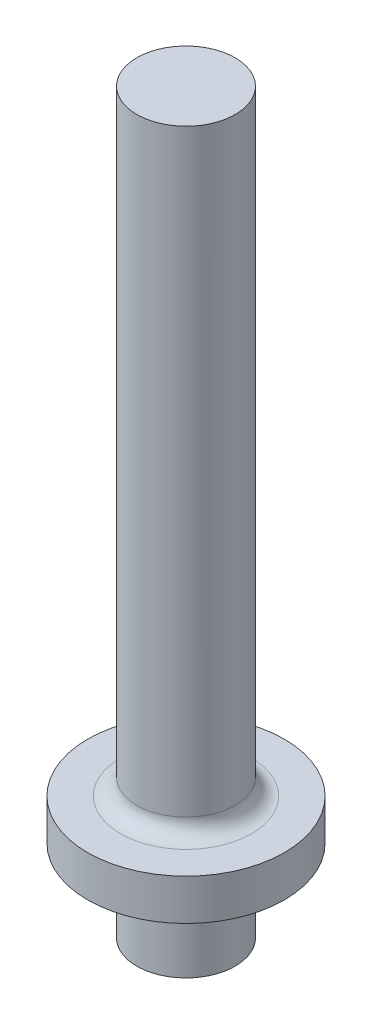
ISO-10303-21;
HEADER;
FILE_DESCRIPTION(('STEP AP214'),'2;1');
FILE_NAME('part.step','',(''),(''),'','','');
FILE_SCHEMA(('AUTOMOTIVE_DESIGN { 1 0 10303 214 1 1 1 1 }'));
ENDSEC;
DATA;
#1=APPLICATION_CONTEXT('core data for automotive mechanical design processes');
#2=APPLICATION_PROTOCOL_DEFINITION('international standard','automotive_design',2000,#1);
#3=PRODUCT_CONTEXT('',#1,'mechanical');
#4=PRODUCT('Part','Part','',(#3));
#5=PRODUCT_RELATED_PRODUCT_CATEGORY('part','',(#4));
#6=PRODUCT_DEFINITION_FORMATION('','',#4);
#7=PRODUCT_DEFINITION_CONTEXT('part definition',#1,'design');
#8=PRODUCT_DEFINITION('design','',#6,#7);
#9=PRODUCT_DEFINITION_SHAPE('','',#8);
#10=(LENGTH_UNIT() NAMED_UNIT(*) SI_UNIT(.MILLI.,.METRE.));
#11=(NAMED_UNIT(*) PLANE_ANGLE_UNIT() SI_UNIT($,.RADIAN.));
#12=(NAMED_UNIT(*) SI_UNIT($,.STERADIAN.) SOLID_ANGLE_UNIT());
#13=UNCERTAINTY_MEASURE_WITH_UNIT(LENGTH_MEASURE(1.E-05),#10,'distance_accuracy_value','');
#14=(GEOMETRIC_REPRESENTATION_CONTEXT(3) GLOBAL_UNCERTAINTY_ASSIGNED_CONTEXT((#13)) GLOBAL_UNIT_ASSIGNED_CONTEXT((#10,
#11,#12)) REPRESENTATION_CONTEXT('',''));
#15=CARTESIAN_POINT('',(0.,0.,0.));
#16=DIRECTION('',(0.,0.,1.));
#17=DIRECTION('',(1.,0.,0.));
#18=AXIS2_PLACEMENT_3D('',#15,#16,#17);
#19=CARTESIAN_POINT('',(0.,0.,0.));
#20=DIRECTION('',(0.,1.,0.));
#21=DIRECTION('',(-1.,0.,0.));
#22=AXIS2_PLACEMENT_3D('',#19,#20,#21);
#23=PLANE('',#22);
#24=CARTESIAN_POINT('',(0.,0.,0.));
#25=DIRECTION('',(0.,1.,0.));
#26=DIRECTION('',(-1.,0.,0.));
#27=AXIS2_PLACEMENT_3D('',#24,#25,#26);
#28=CIRCLE('',#27,6.);
#29=CARTESIAN_POINT('',(-6.,0.,0.));
#30=VERTEX_POINT('',#29);
#31=EDGE_CURVE('E48',#30,#30,#28,.T.);
#32=ORIENTED_EDGE('',*,*,#31,.F.);
#33=EDGE_LOOP('',(#32));
#34=FACE_BOUND('',#33,.T.);
#35=ADVANCED_FACE('F40',(#34),#23,.F.);
#36=CARTESIAN_POINT('',(0.,90.,0.));
#37=DIRECTION('',(0.,1.,0.));
#38=DIRECTION('',(-1.,0.,0.));
#39=AXIS2_PLACEMENT_3D('',#36,#37,#38);
#40=CYLINDRICAL_SURFACE('',#39,6.);
#41=CARTESIAN_POINT('',(0.,9.99999999999999,0.));
#42=DIRECTION('',(0.,1.,0.));
#43=DIRECTION('',(-1.,0.,0.));
#44=AXIS2_PLACEMENT_3D('',#41,#42,#43);
#45=CIRCLE('',#44,6.);
#46=CARTESIAN_POINT('',(-6.,9.99999999999999,0.));
#47=VERTEX_POINT('',#46);
#48=EDGE_CURVE('E55',#47,#47,#45,.T.);
#49=ORIENTED_EDGE('',*,*,#48,.F.);
#50=EDGE_LOOP('',(#49));
#51=FACE_BOUND('',#50,.T.);
#52=ORIENTED_EDGE('',*,*,#31,.T.);
#53=EDGE_LOOP('',(#52));
#54=FACE_BOUND('',#53,.T.);
#55=ADVANCED_FACE('F85',(#51,#54),#40,.T.);
#56=CARTESIAN_POINT('',(12.,10.,0.));
#57=DIRECTION('',(0.,1.,0.));
#58=DIRECTION('',(-1.,0.,0.));
#59=AXIS2_PLACEMENT_3D('',#56,#57,#58);
#60=PLANE('',#59);
#61=CARTESIAN_POINT('',(0.,9.99999999999999,0.));
#62=DIRECTION('',(0.,1.,0.));
#63=DIRECTION('',(-1.,0.,0.));
#64=AXIS2_PLACEMENT_3D('',#61,#62,#63);
#65=CIRCLE('',#64,12.);
#66=CARTESIAN_POINT('',(-12.,9.99999999999999,0.));
#67=VERTEX_POINT('',#66);
#68=EDGE_CURVE('E60',#67,#67,#65,.T.);
#69=ORIENTED_EDGE('',*,*,#68,.F.);
#70=EDGE_LOOP('',(#69));
#71=FACE_BOUND('',#70,.T.);
#72=ORIENTED_EDGE('',*,*,#48,.T.);
#73=EDGE_LOOP('',(#72));
#74=FACE_BOUND('',#73,.T.);
#75=ADVANCED_FACE('F87',(#71,#74),#60,.F.);
#76=CARTESIAN_POINT('',(0.,90.,0.));
#77=DIRECTION('',(0.,1.,0.));
#78=DIRECTION('',(-1.,0.,0.));
#79=AXIS2_PLACEMENT_3D('',#76,#77,#78);
#80=CYLINDRICAL_SURFACE('',#79,12.);
#81=CARTESIAN_POINT('',(0.,15.,0.));
#82=DIRECTION('',(0.,1.,0.));
#83=DIRECTION('',(-1.,0.,0.));
#84=AXIS2_PLACEMENT_3D('',#81,#82,#83);
#85=CIRCLE('',#84,12.);
#86=CARTESIAN_POINT('',(-12.,15.,0.));
#87=VERTEX_POINT('',#86);
#88=EDGE_CURVE('E58',#87,#87,#85,.T.);
#89=ORIENTED_EDGE('',*,*,#88,.F.);
#90=EDGE_LOOP('',(#89));
#91=FACE_BOUND('',#90,.T.);
#92=ORIENTED_EDGE('',*,*,#68,.T.);
#93=EDGE_LOOP('',(#92));
#94=FACE_BOUND('',#93,.T.);
#95=ADVANCED_FACE('F80',(#91,#94),#80,.T.);
#96=CARTESIAN_POINT('',(6.,15.,0.));
#97=DIRECTION('',(0.,-1.,0.));
#98=DIRECTION('',(1.,0.,0.));
#99=AXIS2_PLACEMENT_3D('',#96,#97,#98);
#100=PLANE('',#99);
#101=CARTESIAN_POINT('',(0.,15.,0.));
#102=DIRECTION('',(0.,-1.,0.));
#103=DIRECTION('',(1.,0.,0.));
#104=AXIS2_PLACEMENT_3D('',#101,#102,#103);
#105=CIRCLE('',#104,8.);
#106=CARTESIAN_POINT('',(8.,15.,0.));
#107=VERTEX_POINT('',#106);
#108=EDGE_CURVE('E10',#107,#107,#105,.T.);
#109=ORIENTED_EDGE('',*,*,#108,.T.);
#110=EDGE_LOOP('',(#109));
#111=FACE_BOUND('',#110,.T.);
#112=ORIENTED_EDGE('',*,*,#88,.T.);
#113=EDGE_LOOP('',(#112));
#114=FACE_BOUND('',#113,.T.);
#115=ADVANCED_FACE('F72',(#111,#114),#100,.F.);
#116=CARTESIAN_POINT('',(0.,90.,0.));
#117=DIRECTION('',(0.,1.,0.));
#118=DIRECTION('',(-1.,0.,0.));
#119=AXIS2_PLACEMENT_3D('',#116,#117,#118);
#120=CYLINDRICAL_SURFACE('',#119,6.);
#121=CARTESIAN_POINT('',(0.,17.,0.));
#122=DIRECTION('',(0.,-1.,0.));
#123=DIRECTION('',(1.,0.,0.));
#124=AXIS2_PLACEMENT_3D('',#121,#122,#123);
#125=CIRCLE('',#124,6.);
#126=CARTESIAN_POINT('',(6.,17.,0.));
#127=VERTEX_POINT('',#126);
#128=EDGE_CURVE('E42',#127,#127,#125,.F.);
#129=ORIENTED_EDGE('',*,*,#128,.T.);
#130=EDGE_LOOP('',(#129));
#131=FACE_BOUND('',#130,.T.);
#132=CARTESIAN_POINT('',(0.,90.,0.));
#133=DIRECTION('',(0.,1.,0.));
#134=DIRECTION('',(-1.,0.,0.));
#135=AXIS2_PLACEMENT_3D('',#132,#133,#134);
#136=CIRCLE('',#135,6.00000000000001);
#137=CARTESIAN_POINT('',(-6.00000000000002,90.,0.));
#138=VERTEX_POINT('',#137);
#139=EDGE_CURVE('E62',#138,#138,#136,.T.);
#140=ORIENTED_EDGE('',*,*,#139,.F.);
#141=EDGE_LOOP('',(#140));
#142=FACE_BOUND('',#141,.T.);
#143=ADVANCED_FACE('F69',(#131,#142),#120,.T.);
#144=CARTESIAN_POINT('',(6.,90.,0.));
#145=DIRECTION('',(0.,-1.,0.));
#146=DIRECTION('',(1.,0.,0.));
#147=AXIS2_PLACEMENT_3D('',#144,#145,#146);
#148=PLANE('',#147);
#149=ORIENTED_EDGE('',*,*,#139,.T.);
#150=EDGE_LOOP('',(#149));
#151=FACE_BOUND('',#150,.T.);
#152=ADVANCED_FACE('F70',(#151),#148,.F.);
#153=CARTESIAN_POINT('',(0.,17.,0.));
#154=DIRECTION('',(0.,-1.,0.));
#155=DIRECTION('',(1.,0.,0.));
#156=AXIS2_PLACEMENT_3D('',#153,#154,#155);
#157=TOROIDAL_SURFACE('',#156,8.,2.);
#158=ORIENTED_EDGE('',*,*,#108,.F.);
#159=EDGE_LOOP('',(#158));
#160=FACE_BOUND('',#159,.T.);
#161=ORIENTED_EDGE('',*,*,#128,.F.);
#162=EDGE_LOOP('',(#161));
#163=FACE_BOUND('',#162,.T.);
#164=ADVANCED_FACE('F39',(#160,#163),#157,.F.);
#165=CLOSED_SHELL('',(#35,#55,#75,#95,#115,#143,#152,#164));
#166=MANIFOLD_SOLID_BREP('B2',#165);
#167=ADVANCED_BREP_SHAPE_REPRESENTATION('',(#18,#166),#14);
#168=SHAPE_DEFINITION_REPRESENTATION(#9,#167);
ENDSEC;
END-ISO-10303-21;
